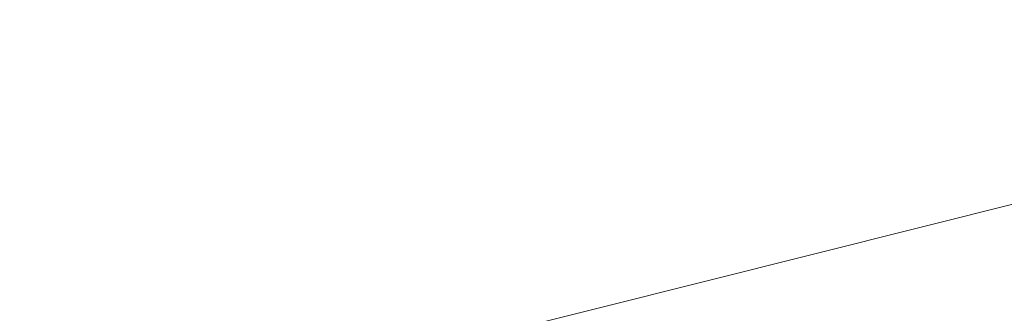
# Model space of a CAD drawing. Units: inches. Extents: x 2091 to 2899, y 967 to 2217.
# Tile 99 of 256: x 2251.243 to 2252.382, y 1100.071 to 1100.41. Entities that reach past the tile are written whole.
import ezdxf

# ---------------------------------------------------------------- set-up
doc = ezdxf.new("R2010")
doc.units = ezdxf.units.IN
doc.layers.add('A-ANNO-DIMS', color=2, linetype='Continuous', lineweight=18)
doc.layers.add('L-PLNT-TREE', color=94, linetype='Continuous', lineweight=13)
doc.layers.add('A-WALL-PATT', color=141, linetype='Continuous', lineweight=13, true_color=0xadddf7)
doc.styles.get("Standard").update_dxf_attribs({"font": 'arial.ttf'})
doc.dimstyles.new('ISO-25', dxfattribs={"dimtxt": 4, "dimasz": 4, "dimexe": 1.25, "dimexo": 0.625, "dimtad": 1, "dimdec": 0, "dimlunit": 3, "dimtxsty": 'Standard', "dimcen": 2.5, "dimadec": 0, "dimazin": 0, "dimtfac": 1, "dimtdec": 0, "dimtmove": 0, "dimatfit": 3, "dimfxl": 1, "dimarcsym": 0})

# ---------------------------------------------------------------- blocks, each defined once
blk = doc.blocks.new('*U29')
blk.add_line((-402.336, 12.192), (-451.104, 0))
blk = doc.blocks.new('*D71')
at = {"layer": 'A-ANNO-DIMS', "color": 0, "lineweight": -2, "transparency": 16777216}
for p, q in [((2212.1436, 1351.2941), (2212.1436, 969.4643)), ((2452.1436, 1351.2941), (2452.1436, 969.4643)), ((2216.1436, 970.7143), (2448.1436, 970.7143))]:
    blk.add_line(p, q, dxfattribs=at)
at = {"layer": 'A-ANNO-DIMS', "color": 0, "transparency": 16777216}
for points in [[(2216.1436, 971.381), (2216.1436, 970.0476), (2212.1436, 970.7143)], [(2448.1436, 971.381), (2448.1436, 970.0476), (2452.1436, 970.7143)]]:
    blk.add_solid(points, dxfattribs=at)
at = {"layer": 'Defpoints', "color": 0, "transparency": 16777216}
for p in [(2212.1436, 1351.9191), (2452.1436, 1351.9191), (2452.1436, 970.7143)]:
    blk.add_point(p, dxfattribs=at)
at = {"layer": 'A-ANNO-DIMS', "color": 0, "transparency": 16777216, "insert": (2332.1436, 973.3816), "char_height": 4, "attachment_point": 5}
blk.add_mtext('20\'-0"', dxfattribs=at)
blk = doc.blocks.new('*D75')
at = {"layer": 'A-ANNO-DIMS', "color": 0, "lineweight": -2, "transparency": 16777216}
for p, q in [((2212.1436, 1274.7941), (2212.1436, 969.4643)), ((2308.1436, 1274.7941), (2308.1436, 969.4643)), ((2216.1436, 970.7143), (2304.1436, 970.7143))]:
    blk.add_line(p, q, dxfattribs=at)
at = {"layer": 'A-ANNO-DIMS', "color": 0, "transparency": 16777216}
for points in [[(2216.1436, 971.381), (2216.1436, 970.0476), (2212.1436, 970.7143)], [(2304.1436, 971.381), (2304.1436, 970.0476), (2308.1436, 970.7143)]]:
    blk.add_solid(points, dxfattribs=at)
at = {"layer": 'Defpoints', "color": 0, "transparency": 16777216}
for p in [(2212.1436, 1275.4191), (2308.1436, 1275.4191), (2308.1436, 970.7143)]:
    blk.add_point(p, dxfattribs=at)
at = {"layer": 'A-ANNO-DIMS', "color": 0, "transparency": 16777216, "insert": (2260.1436, 973.3816), "char_height": 4, "attachment_point": 5}
blk.add_mtext('8\'-0"', dxfattribs=at)

msp = doc.modelspace()

# ---------------------------------------------------------------- hatches: boundary and pattern name
at = {"layer": 'A-WALL-PATT'}
h = msp.add_hatch(color=256, dxfattribs=at)
h.dxf.hatch_style = 1
h.paths.add_polyline_path([(2803.1436, 2050.9191), (2203.1436, 2050.9191), (2203.1436, 1090.9191), (2803.1436, 1090.9191)])
h.paths.add_polyline_path([(2635.7989, 1147.5405), (2674.5241, 1147.5405, 0.376086), (2678.5297, 1152.8802), (2678.5297, 1159.5565, 0.333335), (2674.5243, 1163.5618), (2674.5243, 1163.5619), (2674.5243, 1192.9344), (2635.806, 1192.9344), (2597.0876, 1192.9344), (2597.0876, 1163.5618, 0.333335), (2593.0823, 1159.5565), (2593.0823, 1152.8802, 0.376086), (2597.0879, 1147.5405)], flags=0)
h.paths.add_polyline_path([(2436.0104, 1278.2408, 0.000483), (2435.9526, 1278.215, -0.001328), (2435.9356, 1278.1117, -0.001711), (2436.1164, 1278.0408, 0.002185)], flags=0)
h.paths.add_polyline_path([(2794.1436, 1143.4191), (2794.1436, 1347.4191), (2543.3702, 1347.4191), (2543.3702, 1351.9191), (2794.1436, 1351.9191), (2794.1436, 1392.7136), (2793.9474, 1392.7136), (2793.9474, 1473.5369), (2794.1436, 1473.5369), (2794.1436, 1531.9191), (2650.1436, 1531.9191), (2650.1436, 1536.4191), (2794.1436, 1536.4191), (2794.1436, 1692.4191), (2609.3756, 1692.4191), (2609.3756, 1644.4191), (2604.8756, 1644.4191), (2604.8756, 1744.9191), (2609.3756, 1744.9191), (2609.3756, 1696.9191), (2794.1436, 1696.9191), (2794.1436, 1780.9191), (2609.6436, 1780.9191), (2493.8756, 1780.9191), (2493.8756, 1785.4191), (2609.6436, 1785.4191), (2794.1436, 1785.4191), (2794.1436, 1847.9388), (2793.9512, 1847.9388), (2793.9512, 1928.7622), (2794.1436, 1928.7622), (2794.1436, 1941.4191), (2614.1436, 1941.4191), (2614.1436, 1821.4191), (2609.6436, 1821.4191), (2609.6436, 1941.4191), (2392.1436, 1941.4191), (2392.1436, 1819.9191), (2387.6436, 1819.9191), (2387.6436, 1941.4191), (2212.1436, 1941.4191), (2212.1436, 1783.9191), (2392.1436, 1783.9191), (2392.1436, 1780.9191), (2212.1436, 1780.9191), (2212.1436, 1629.4191), (2387.6436, 1629.4191), (2387.6436, 1744.9191), (2392.1436, 1744.9191), (2392.1436, 1627.9191), (2317.1436, 1627.9191), (2317.1436, 1551.4191), (2317.1436, 1536.4191), (2459.3836, 1536.4191), (2459.3836, 1602.3965), (2463.8836, 1602.3965), (2463.8836, 1531.9191), (2456.6436, 1531.9191), (2456.6436, 1529.9191), (2452.1436, 1529.9191), (2452.1436, 1531.9191), (2312.6436, 1531.9191), (2312.6436, 1551.4191), (2306.1436, 1551.4191), (2306.1436, 1555.9191), (2308.1436, 1555.9191), (2308.1436, 1551.4191), (2312.6436, 1551.4191), (2312.6436, 1627.9191), (2212.1436, 1627.9191), (2212.1436, 1555.9191), (2270.1436, 1555.9191), (2270.1436, 1551.4191), (2212.1436, 1551.4191), (2212.1436, 1351.9191), (2272.1436, 1351.9191), (2272.1436, 1347.4191), (2212.1436, 1347.4191), (2212.1436, 1275.4191), (2308.1436, 1275.4191), (2308.1436, 1351.9191), (2452.1436, 1351.9191), (2452.1436, 1493.9191), (2456.6436, 1493.9191), (2456.6436, 1347.4191), (2312.6436, 1347.4191), (2312.6436, 1270.9191), (2212.1436, 1270.9191), (2212.1436, 1099.9191), (2281.2375, 1099.9191), (2282.871, 1110.9138), (2282.0083, 1116.9966), (2278.5577, 1121.4204), (2268.2056, 1128.0562), (2272.0876, 1128.0562), (2273.8129, 1131.927), (2279.4203, 1134.6919), (2285.0278, 1135.2449), (2287.6158, 1137.4568), (2288.0471, 1138.0098), (2289.3411, 1140.7747), (2291.0665, 1139.6687), (2292.3605, 1135.2449), (2295.3798, 1136.9038), (2296.2425, 1135.7979), (2297.1052, 1133.033), (2300.1246, 1138.0098), (2303.1439, 1138.0098), (2304.4379, 1135.7979), (2303.1439, 1133.586), (2306.5946, 1134.6919), (2307.8887, 1133.033), (2310.908, 1135.2449), (2313.9274, 1134.1389), (2315.6269, 1132.4271), (2308.32, 1117.5496), (2290.2038, 1109.8079), (2288.9098, 1103.1721), (2289.2723, 1099.9191), (2434.9182, 1099.9191), (2431.5932, 1124.7881), (2429.9302, 1169.5531), (2430.9272, 1240.5197), (2435.6589, 1238.1861), (2437.1352, 1196.5541), (2438.7982, 1143.9731), (2442.6782, 1111.9981), (2446.5582, 1099.9191), (2794.1436, 1099.9191), (2794.1436, 1138.9191), (2548.0324, 1138.9191), (2548.0324, 1143.4191), (2548.0324, 1148.8191), (2546.6685, 1148.0316), (2528.6857, 1179.1786, 0.256256), (2512.0324, 1148.8191), (2512.0324, 1143.4191), (2512.0324, 1138.9191), (2507.5324, 1138.9191), (2507.5324, 1143.4191), (2507.5324, 1148.8191, 0.256256), (2490.8792, 1179.1786), (2472.8964, 1148.0316), (2471.5324, 1148.8191), (2471.5324, 1143.4191), (2467.0324, 1143.4191), (2467.0324, 1269.9458, 0.039061), (2460.91, 1273.5801), (2467.0324, 1273.5801), (2467.0324, 1286.3254, 0.014511), (2465.2162, 1286.7619), (2467.0324, 1287.0526), (2467.0324, 1323.4191), (2471.5324, 1323.4191), (2471.5324, 1148.8191), (2489.5324, 1179.996), (2490.8964, 1179.2085), (2490.8792, 1179.1786, -0.256256), (2507.5324, 1148.8191), (2507.5324, 1143.4191), (2512.0324, 1143.4191), (2512.0324, 1148.8191, -0.256256), (2528.6857, 1179.1786), (2528.6685, 1179.2085), (2530.0324, 1179.996), (2548.0324, 1148.8191), (2548.0324, 1143.4191)], flags=16)
h.paths.add_polyline_path([(2607.7685, 1200.9451), (2607.7685, 1265.0306), (2597.0876, 1281.052), (2619.7846, 1281.052), (2627.7953, 1337.1269), (2635.7989, 1337.1269), (2643.8167, 1337.1269), (2651.8274, 1281.052), (2674.5243, 1281.052), (2663.8434, 1265.0306), (2663.8434, 1200.9451), (2635.806, 1200.9451)], flags=0)
edge = h.paths.add_edge_path(flags=0)
edge.add_ellipse((13303.8962, 1272.9987), major_axis=(-10595.313, 0), ratio=0.8423038701, start_angle=0.62823722, end_angle=0.6465541, ccw=False)
edge.add_ellipse((2711.7004, 1156.8527), major_axis=(2.2198, 0), ratio=0.842304, start_angle=111.5352, end_angle=180.6282, ccw=False)
edge.add_ellipse((13303.1563, 1272.9987), major_axis=(-10593.0263, 0), ratio=0.8423038695, start_angle=0.52827147, end_angle=0.6465541, ccw=False)
edge.add_line((2710.7646, 1175.3333), (2710.13, 1175.3333))
edge.add_ellipse((2710.13, 1176.5798), major_axis=(1.4798, 0), ratio=0.842304, start_angle=180, end_angle=270, ccw=False)
edge.add_line((2708.6501, 1176.5798), (2708.6501, 1200.7829))
edge.add_ellipse((2710.13, 1200.7829), major_axis=(1.4798, 0), ratio=0.842304, start_angle=90, end_angle=180, ccw=False)
edge.add_line((2710.13, 1202.0294), (2710.4651, 1202.0294))
edge.add_ellipse((13303.1563, 1272.9987), major_axis=(-10593.0263, 0), ratio=0.8423038695, start_angle=-0.09022909, end_angle=0.38386678, ccw=False)
edge.add_ellipse((2710.13, 1290.927), major_axis=(-1.4798, 0), ratio=0.842304, start_angle=0, end_angle=90, ccw=False)
edge.add_line((2708.6501, 1290.927), (2708.6501, 1315.1302))
edge.add_ellipse((2710.13, 1315.1302), major_axis=(-1.4798, 0), ratio=0.842304, start_angle=-90, end_angle=0, ccw=False)
edge.add_line((2710.13, 1316.3767), (2710.7063, 1316.3767))
edge.add_ellipse((3238.4017, 1296.2896), major_axis=(528.234, 0), ratio=0.84230387, start_angle=176.349572, end_angle=177.82005, ccw=False)
edge.add_ellipse((2775.063, 1071.4507), major_axis=(313.3078, 0), ratio=0.84230387, start_angle=102.125966, end_angle=103.780529, ccw=False)
edge.add_ellipse((2775.063, 1078.3057), major_axis=(-305.3029, 0), ratio=0.84230387, start_angle=-79.790461, end_angle=-77.555373, ccw=False)
edge.add_ellipse((2695.1418, 1541.9754), major_axis=(-250.9602, 0), ratio=0.84230387, start_angle=99.256566, end_angle=102.554933)
edge.add_line((2741.4103, 1334.2143), (2747.1325, 1337.3785))
edge.add_ellipse((2747.5386, 1336.8575), major_axis=(-0.7399, 0), ratio=0.842304, start_angle=270, end_angle=307.9331, ccw=False)
edge.add_ellipse((2747.5386, 1336.8575), major_axis=(-0.7399, 0), ratio=0.842304, start_angle=232.0669, end_angle=270, ccw=False)
edge.add_line((2747.9447, 1337.3785), (2753.6669, 1334.2143))
edge.add_ellipse((2799.9355, 1541.9754), major_axis=(250.9602, 0), ratio=0.84230387, start_angle=257.445067, end_angle=260.743434)
edge.add_ellipse((2720.0142, 1078.3057), major_axis=(305.3029, 0), ratio=0.84230387, start_angle=77.555373, end_angle=79.790461, ccw=False)
edge.add_ellipse((2720.0142, 1071.4507), major_axis=(-313.3078, 0), ratio=0.84230387, start_angle=256.219471, end_angle=257.874034, ccw=False)
edge.add_ellipse((2256.6755, 1296.2896), major_axis=(-528.234, 0), ratio=0.84230387, start_angle=182.17995, end_angle=183.650428, ccw=False)
edge.add_line((2784.3709, 1316.3767), (2784.9472, 1316.3767))
edge.add_ellipse((2784.9472, 1315.1302), major_axis=(1.4798, 0), ratio=0.842304, start_angle=0, end_angle=90, ccw=False)
edge.add_line((2786.4271, 1315.1302), (2786.4271, 1290.927))
edge.add_ellipse((2784.9472, 1290.927), major_axis=(1.4798, 0), ratio=0.842304, start_angle=270, end_angle=360, ccw=False)
edge.add_ellipse((-7808.0791, 1272.9987), major_axis=(10593.0263, 0), ratio=0.8423038695, start_angle=-0.38386678, end_angle=0.09022909, ccw=False)
edge.add_line((2784.6122, 1202.0294), (2784.9472, 1202.0294))
edge.add_ellipse((2784.9472, 1200.7829), major_axis=(1.4798, 0), ratio=0.842304, start_angle=0, end_angle=90, ccw=False)
edge.add_line((2786.4271, 1200.7829), (2786.4271, 1176.5798))
edge.add_ellipse((2784.9472, 1176.5798), major_axis=(-1.4798, 0), ratio=0.842304, start_angle=90, end_angle=180, ccw=False)
edge.add_line((2784.9472, 1175.3333), (2784.3126, 1175.3333))
edge.add_ellipse((-7808.0791, 1272.9987), major_axis=(10593.0263, 0), ratio=0.8423038695, start_angle=-0.6186432, end_angle=-0.52827147, ccw=False)
edge.add_ellipse((2783.3768, 1156.8527), major_axis=(-2.2198, 0), ratio=0.842304, start_angle=179.3718, end_angle=248.4648, ccw=False)
edge.add_ellipse((-7808.819, 1272.9987), major_axis=(-10595.313, 0), ratio=0.8423038658, start_angle=179.35344592, end_angle=179.3717628, ccw=False)
edge.add_ellipse((2780.2973, 1153.5008), major_axis=(-5.2464, 0), ratio=0.842304, start_angle=90, end_angle=179.3534, ccw=False)
edge.add_line((2780.2973, 1149.0817), (2714.7799, 1149.0817))
edge.add_ellipse((2714.7799, 1153.5008), major_axis=(5.2464, 0), ratio=0.842304, start_angle=180.6466, end_angle=270, ccw=False)
edge = h.paths.add_edge_path(flags=0)
edge.add_line((2718.1874, 1151.0078), (2718.1874, 1170.4724))
edge.add_ellipse((2721.1471, 1170.4724), major_axis=(-2.9597, 0), ratio=0.842304, start_angle=-90, end_angle=0, ccw=False)
edge.add_line((2721.1471, 1172.9653), (2773.9302, 1172.9653))
edge.add_ellipse((2773.9302, 1170.4724), major_axis=(-2.9597, 0), ratio=0.842304, start_angle=180, end_angle=270, ccw=False)
edge.add_line((2776.8899, 1170.4724), (2776.8899, 1151.0078))
edge.add_line((2776.8899, 1151.0078), (2718.1874, 1151.0078))
edge = h.paths.add_edge_path(flags=0)
edge.add_line((2718.1874, 1180.2342), (2718.1874, 1199.0578))
edge.add_ellipse((2747.5386, 1320.3986), major_axis=(147.0179, 0), ratio=0.84230387, start_angle=256.401865, end_angle=283.598135)
edge.add_line((2776.8899, 1199.0578), (2776.8899, 1180.2342))
edge.add_ellipse((2747.5386, 1301.575), major_axis=(147.0179, 0), ratio=0.84230387, start_angle=256.401865, end_angle=283.598135, ccw=False)
edge = h.paths.add_edge_path(flags=0)
edge.add_ellipse((13303.1563, 1272.9987), major_axis=(-10591.5465, 0), ratio=0.8423038696, start_angle=0.05559431, end_angle=0.37776419, ccw=False)
edge.add_line((2711.6169, 1262.7217), (2715.6674, 1249.4954))
edge.add_ellipse((6413.892, 1241.6919), major_axis=(-3698.2362, 0), ratio=0.84230387, start_angle=-0.1208974, end_angle=0.3640763)
edge.add_line((2715.761, 1218.1925), (2711.9343, 1203.1674))
edge = h.paths.add_edge_path(flags=0)
edge.add_line((2718.1874, 1251.0746), (2716.0025, 1267.4504))
edge.add_ellipse((2742.1512, 1202.1895), major_axis=(81.7726, 0), ratio=0.8423039, start_angle=94.277421, end_angle=111.834954, ccw=False)
edge.add_line((2737.0097, 1270.9306), (2758.0675, 1270.9306))
edge.add_ellipse((2752.9261, 1202.1895), major_axis=(81.7726, 0), ratio=0.8423039, start_angle=68.165046, end_angle=85.722579, ccw=False)
edge.add_line((2779.0747, 1267.4504), (2776.8899, 1251.0746))
edge.add_ellipse((2750.3381, 1187.8854), major_axis=(79.5797, 0), ratio=0.8423039, start_angle=67.208085, end_angle=85.12993)
edge.add_line((2756.0347, 1254.7437), (2739.0426, 1254.7437))
edge.add_ellipse((2744.7392, 1187.8854), major_axis=(79.5797, 0), ratio=0.8423039, start_angle=94.87007, end_angle=112.791915)
edge = h.paths.add_edge_path(flags=0)
edge.add_line((2783.1429, 1203.1674), (2779.3162, 1218.1925))
edge.add_ellipse((-918.8147, 1241.6919), major_axis=(3698.2362, 0), ratio=0.84230387, start_angle=-0.3640763, end_angle=0.1208974)
edge.add_line((2779.4098, 1249.4954), (2783.4604, 1262.7217))
edge.add_ellipse((-7808.0791, 1272.9987), major_axis=(-10591.5465, 0), ratio=0.8423038695, start_angle=179.62223581, end_angle=179.94440569, ccw=False)
edge = h.paths.add_edge_path(flags=0)
edge.add_ellipse((2734.2009, 1286.6904), major_axis=(-0.3566, 6.3401), ratio=0.603834, start_angle=89.00201, end_angle=253.65741, ccw=False)
edge.add_line((2730.369, 1286.5418), (2730.369, 1301.352))
edge.add_line((2730.369, 1301.352), (2735.9133, 1305.2148))
edge.add_ellipse((2736.3849, 1304.7346), major_axis=(0.7399, 0), ratio=0.842304, start_angle=90, end_angle=134.4802, ccw=False)
edge.add_line((2736.3849, 1305.3578), (2738.0328, 1305.3578))
edge.add_line((2738.0328, 1305.3578), (2738.0328, 1307.7079))
edge.add_ellipse((2794.2016, 1307.7079), major_axis=(56.1689, 0), ratio=0.8423039, start_angle=150.56143, end_angle=180, ccw=False)
edge.add_ellipse((2700.8756, 1307.7079), major_axis=(-56.1689, 0), ratio=0.8423039, start_angle=180, end_angle=209.43857, ccw=False)
edge.add_line((2757.0444, 1307.7079), (2757.0444, 1305.3578))
edge.add_line((2757.0444, 1305.3578), (2758.6923, 1305.3578))
edge.add_ellipse((2758.6923, 1304.7346), major_axis=(-0.7399, 0), ratio=0.842304, start_angle=225.5198, end_angle=270, ccw=False)
edge.add_line((2759.1639, 1305.2148), (2764.7082, 1301.352))
edge.add_line((2764.7082, 1301.352), (2764.7082, 1286.5418))
edge.add_ellipse((2760.8763, 1286.6904), major_axis=(0.3566, 6.3401), ratio=0.603834, start_angle=106.34259, end_angle=270.99799, ccw=False)
edge.add_line((2757.0444, 1285.7971), (2757.0444, 1307.7079))
edge.add_ellipse((2700.8756, 1307.7079), major_axis=(-56.1689, 0), ratio=0.8423039, start_angle=180, end_angle=209.43857)
edge.add_ellipse((2794.2016, 1307.7079), major_axis=(56.1689, 0), ratio=0.8423039, start_angle=150.56143, end_angle=180)
edge.add_line((2738.0328, 1307.7079), (2738.0328, 1285.7971))
h.paths.add_polyline_path([(2417.8123, 1104.4497), (2413.4923, 1102.5297), (2410.6123, 1103.9697), (2409.1723, 1106.3697), (2407.2523, 1107.3297), (2406.2923, 1109.7297), (2405.3323, 1114.0497), (2405.3323, 1117.8897), (2406.2923, 1120.1297), (2407.2523, 1119.8097), (2408.8483, 1118.3277), (2410.1739, 1119.4242), (2410.2113, 1120.4057), (2411.0407, 1121.4191), (2410.6993, 1119.8587), (2410.1739, 1119.4242), (2410.0885, 1117.1761), (2411.1328, 1116.2063), (2413.9723, 1119.3297), (2416.8523, 1120.7697), (2416.8697, 1120.7988), (2417.0351, 1119.4051), (2417.8962, 1118.1434), (2418.2923, 1118.3697), (2419.5444, 1120.0393), (2419.3609, 1118.3875), (2419.0321, 1119.3562), (2418.3989, 1118.5119), (2419.2523, 1114.5297), (2418.7941, 1107.1988)], flags=0)
h.paths.add_polyline_path([(2508.8702, 1347.4191), (2508.3702, 1347.4191), (2508.3702, 1351.9191), (2508.8702, 1351.9191)], flags=0)
h.paths.add_polyline_path([(2473.3702, 1347.4191), (2472.3702, 1347.4191), (2467.8702, 1347.4191), (2467.8702, 1455.4191), (2472.3702, 1455.4191), (2472.3702, 1352.4191), (2473.3702, 1352.4191)], flags=0)
h.paths.add_polyline_path([(2352.1062, 1217.4462), (2349.2262, 1218.8862), (2347.7862, 1221.2862), (2345.8662, 1222.2462), (2344.9062, 1224.6462), (2343.9462, 1228.9662), (2343.9462, 1232.8062), (2344.9062, 1235.0462), (2345.8662, 1234.7262), (2347.4623, 1233.2442), (2348.7879, 1234.3407), (2348.8252, 1235.3222), (2349.6547, 1236.3355), (2349.3132, 1234.7752), (2348.7879, 1234.3407), (2348.7024, 1232.0926), (2349.7468, 1231.1228), (2352.5862, 1234.2462), (2355.4662, 1235.6862), (2355.4837, 1235.7153), (2355.649, 1234.3216), (2356.5102, 1233.0599), (2356.9062, 1233.2862), (2358.1584, 1234.9558), (2357.9749, 1233.304), (2357.6461, 1234.2726), (2357.0129, 1233.4284), (2357.8662, 1229.4462), (2357.4081, 1222.1153), (2356.4262, 1219.3662)], flags=0)
h.paths.add_polyline_path([(2348.2968, 1112.2244), (2347.0138, 1112.3104), (2345.5298, 1114.1274), (2345.7318, 1115.8584), (2346.8118, 1116.9824), (2346.8118, 1114.6464), (2345.8668, 1114.2144), (2346.8798, 1114.3004)], flags=0)
h.paths.add_polyline_path([(2347.0138, 1110.9264), (2346.2718, 1110.4934), (2346.6098, 1111.1864)], flags=0)
h.paths.add_polyline_path([(2345.8668, 1118.1944), (2345.5298, 1117.3294), (2343.7078, 1118.0214), (2344.3828, 1118.6264)], flags=0)
h.paths.add_polyline_path([(2346.6768, 1109.2824), (2346.0698, 1108.0714), (2345.8668, 1110.0614)], flags=0)
h.paths.add_polyline_path([(2345.0568, 1119.7514), (2343.6398, 1119.7514), (2343.9778, 1121.1354)], flags=0)
h.paths.add_polyline_path([(2345.2598, 1116.5504), (2345.1248, 1115.8584), (2344.9218, 1115.6854), (2344.7198, 1116.3774)], flags=0)
h.paths.add_polyline_path([(2345.6648, 1112.3104), (2345.4618, 1111.5324), (2344.0448, 1111.9644), (2344.6518, 1112.5704)], flags=0)
h.paths.add_polyline_path([(2345.1918, 1113.3494), (2344.4498, 1113.8684), (2344.7198, 1114.3874)], flags=0)
h.paths.add_polyline_path([(2344.6518, 1116.8094), (2344.1798, 1115.6854), (2344.6518, 1115.3394), (2343.9098, 1114.9064), (2343.0328, 1115.9444), (2343.6398, 1116.4634)], flags=0)
h.paths.add_polyline_path([(2345.8668, 1106.6864), (2344.9898, 1105.5624), (2344.5168, 1106.6004)], flags=0)
h.paths.add_polyline_path([(2344.8548, 1110.0614), (2344.5168, 1109.2824), (2344.1128, 1109.7154)], flags=0)
h.paths.add_polyline_path([(2344.0448, 1113.5224), (2343.4378, 1113.0894), (2342.7628, 1113.9544)], flags=0)
h.paths.add_polyline_path([(2344.3148, 1111.0124), (2342.9648, 1110.3204), (2342.9648, 1111.0994)], flags=0)
h.paths.add_polyline_path([(2345.1248, 1104.6974), (2344.5848, 1103.7454), (2344.4498, 1104.2644)], flags=0)
h.paths.add_polyline_path([(2342.8298, 1121.2224), (2341.7498, 1120.5304), (2340.5358, 1121.0494), (2340.1308, 1121.8284), (2340.6708, 1122.9524), (2341.1428, 1121.8284), (2341.6148, 1122.0014)], flags=0)
h.paths.add_polyline_path([(2342.9648, 1119.7514), (2343.0328, 1118.4534), (2342.0878, 1118.0214), (2342.0198, 1119.4914)], flags=0)
h.paths.add_polyline_path([(2342.6948, 1116.8964), (2341.9528, 1116.6364), (2342.0198, 1117.3294)], flags=0)
h.paths.add_polyline_path([(2343.0328, 1112.2244), (2342.0198, 1111.7914), (2341.5478, 1112.2244), (2342.3578, 1113.3494)], flags=0)
h.paths.add_polyline_path([(2343.7748, 1104.4374), (2342.6278, 1102.8804), (2342.6948, 1104.6104), (2343.4378, 1105.1294)], flags=0)
h.paths.add_polyline_path([(2342.0198, 1115.0794), (2340.8058, 1115.5124), (2340.9408, 1116.3774)], flags=0)
h.paths.add_polyline_path([(2341.4808, 1120.0974), (2341.4808, 1119.4054), (2341.0758, 1119.5784), (2341.1428, 1120.0974)], flags=0)
h.paths.add_polyline_path([(2341.8178, 1114.4734), (2340.9408, 1113.0894), (2340.8058, 1114.5604)], flags=0)
h.paths.add_polyline_path([(2341.1428, 1118.5404), (2340.9408, 1116.9824), (2339.0508, 1117.6754), (2339.0508, 1118.6264)], flags=0)
h.paths.add_polyline_path([(2342.6948, 1101.6684), (2341.9528, 1101.8414), (2342.5598, 1102.3614)], flags=0)
h.paths.add_polyline_path([(2340.3328, 1119.6654), (2338.4438, 1119.5784), (2337.9038, 1120.3574), (2339.6578, 1120.6164)], flags=0)
h.paths.add_polyline_path([(2340.3328, 1115.3394), (2340.0628, 1113.6954), (2339.3878, 1115.3394)], flags=0)
h.paths.add_polyline_path([(2341.8178, 1103.8314), (2341.5478, 1102.8804), (2341.1428, 1103.6584)], flags=0)
h.paths.add_polyline_path([(2339.0508, 1122.8664), (2337.2958, 1121.8284), (2337.0938, 1123.1254), (2337.7688, 1123.8184)], flags=0)
h.paths.add_polyline_path([(2339.1178, 1121.7414), (2338.8478, 1121.2224), (2338.1738, 1121.0494), (2338.3758, 1121.5684)], flags=0)
h.paths.add_polyline_path([(2339.1858, 1119.3194), (2338.6458, 1118.7134), (2338.2408, 1118.1074), (2338.2408, 1118.8864)], flags=0)
h.paths.add_polyline_path([(2341.1428, 1101.9284), (2340.6028, 1101.2364), (2340.0628, 1101.8414), (2340.6028, 1102.3614)], flags=0)
h.paths.add_polyline_path([(2337.6338, 1117.7614), (2336.6208, 1118.2804), (2337.2958, 1118.9724)], flags=0)
h.paths.add_polyline_path([(2336.8238, 1119.5784), (2334.7988, 1118.9724), (2335.2038, 1120.3574), (2336.5538, 1120.8764)], flags=0)
h.paths.add_polyline_path([(2339.1178, 1100.4574), (2337.3638, 1100.5434), (2336.7558, 1101.2364)], flags=0)
h.paths.add_polyline_path([(2336.3508, 1122.4334), (2336.0138, 1121.9144), (2334.9338, 1122.4334), (2334.5288, 1123.4714), (2335.7438, 1122.7794)], flags=0)
h.paths.add_polyline_path([(2334.7318, 1120.8764), (2334.2588, 1120.3574), (2334.0568, 1120.7894), (2334.5968, 1121.3084)], flags=0)
h.paths.add_polyline_path([(2334.4618, 1122.1744), (2332.5718, 1121.3084), (2331.3568, 1122.1744), (2332.0998, 1122.8664)], flags=0)
h.paths.add_polyline_path([(2334.2588, 1118.5404), (2333.3818, 1118.4534), (2333.6518, 1119.3194)], flags=0)
h.paths.add_polyline_path([(2335.5418, 1102.2744), (2334.1918, 1102.6204), (2335.2718, 1103.3124)], flags=0)
h.paths.add_polyline_path([(2332.7068, 1119.6654), (2331.6948, 1120.4434), (2332.5048, 1120.7894)], flags=0)
h.paths.add_polyline_path([(2334.7318, 1101.1494), (2333.5168, 1101.5824), (2333.9888, 1101.7554)], flags=0)
h.paths.add_polyline_path([(2332.6398, 1116.6364), (2331.0868, 1116.2904), (2331.9648, 1118.1944)], flags=0)
h.paths.add_polyline_path([(2330.7498, 1121.5684), (2330.2768, 1120.2704), (2328.5228, 1119.3194), (2328.9948, 1121.0494)], flags=0)
h.paths.add_polyline_path([(2330.7498, 1118.6264), (2330.0078, 1117.5024), (2329.8728, 1118.0214)], flags=0)
h.paths.add_polyline_path([(2332.0998, 1102.3614), (2330.5468, 1102.0144), (2331.6948, 1102.9664)], flags=0)
h.paths.add_polyline_path([(2329.5348, 1113.6084), (2329.0628, 1112.3104), (2328.5898, 1113.3494)], flags=0)
h.paths.add_polyline_path([(2328.3878, 1117.8484), (2327.5098, 1116.5504), (2327.1728, 1117.7614)], flags=0)
h.paths.add_polyline_path([(2329.7378, 1106.5134), (2329.5348, 1105.3024), (2328.2528, 1106.0814)], flags=0)
h.paths.add_polyline_path([(2328.6578, 1114.3874), (2328.0498, 1114.1274), (2328.3198, 1114.9064)], flags=0)
h.paths.add_polyline_path([(2328.3198, 1112.2244), (2327.1058, 1112.1374), (2326.7008, 1112.6564)], flags=0)
h.paths.add_polyline_path([(2326.9028, 1115.2524), (2326.7008, 1114.1274), (2325.2158, 1113.6084), (2326.0928, 1115.3394)], flags=0)
h.paths.add_polyline_path([(2326.6328, 1108.3304), (2326.0928, 1107.3794), (2325.8908, 1108.5034), (2326.4978, 1109.1094)], flags=0)
h.paths.add_polyline_path([(2615.1436, 1531.9191), (2609.6436, 1531.9191), (2609.6436, 1620.4191), (2614.1436, 1620.4191), (2614.1436, 1536.4191), (2615.1436, 1536.4191)], flags=0)
h.paths.add_polyline_path([(2545.1436, 1563.4191), (2464.1436, 1563.4191), (2464.1436, 1632.4191), (2509.1436, 1632.4191), (2509.1436, 1627.9191), (2509.1436, 1603.9191), (2468.6436, 1603.9191), (2468.6436, 1567.9191), (2540.6436, 1567.9191), (2540.6436, 1591.9191), (2545.1436, 1591.9191)], flags=0)
h.paths.add_polyline_path([(2388.969, 1549.9857), (2357.4342, 1549.9857), (2357.4342, 1623.3608), (2399.3628, 1623.3608), (2435.6895, 1623.3608), (2435.5925, 1602.5593), (2435.5925, 1602.3965), (2388.969, 1602.3965)], flags=0)
h.paths.add_polyline_path([(2388.8806, 1555.8092), (2374.9044, 1555.8092), (2374.9044, 1600.5716), (2374.9044, 1615.4576), (2406.3509, 1615.4576), (2406.3509, 1618.9394), (2412.1743, 1615.4576), (2406.3509, 1611.9759), (2406.3509, 1615.4576), (2388.8806, 1615.4576)], flags=0)
h.paths.add_polyline_path([(2568.8756, 1644.4191), (2453.3756, 1644.4191), (2453.3756, 1785.4191), (2457.8756, 1785.4191), (2457.8756, 1648.9191), (2568.8756, 1648.9191)], flags=0)
h.paths.add_polyline_path([(2212.1436, 1945.9191), (2212.1436, 2041.9191), (2794.1436, 2041.9191), (2794.1436, 1945.9191)], flags=16)
h.paths.add_polyline_path([(2271.0827, 1964.3172), (2776.853, 1964.3172), (2776.853, 2037.1696), (2271.0827, 2037.1696)], flags=8)
h.paths.add_polyline_path([(2380.6493, 1536.8241), (2461.0408, 1536.8241), (2461.0408, 1554.6526), (2380.6493, 1554.6526)], flags=8)
h.paths.add_polyline_path([(2240.7557, 1609.7255), (2309.1858, 1609.7255), (2309.1858, 1617.6982), (2240.7557, 1617.6982)], flags=8)
h.paths.add_polyline_path([(2212.6773, 1313.5041), (2282.5915, 1313.5041), (2282.5915, 1322.7452), (2212.6773, 1322.7452)], flags=8)
h.paths.add_polyline_path([(2457.112, 1114.7786), (2558.4816, 1114.7786), (2558.4816, 1142.2197), (2457.112, 1142.2197)], flags=8)
h.paths.add_polyline_path([(2473.4423, 1273.0101), (2604.6412, 1273.0101), (2604.6412, 1318.3469), (2473.4423, 1318.3469)], flags=8)
h.paths.add_polyline_path([(2638.8763, 1626.9774), (2684.2504, 1627.9767), (2684.0385, 1637.5975), (2638.6644, 1636.5982)], flags=8)
h.paths.add_polyline_path([(2537.5906, 1453.7934), (2628.3895, 1453.7934), (2628.3895, 1475.3448), (2537.5906, 1475.3448)], flags=8)
h.paths.add_polyline_path([(2504.1376, 1714.6324), (2554.6472, 1714.6324), (2554.6472, 1730.2377), (2504.1376, 1730.2377)], flags=8)
h.paths.add_polyline_path([(2487.5012, 1575.6519), (2535.0971, 1575.6519), (2535.0971, 1598.3776), (2487.5012, 1598.3776)], flags=8)
h.paths.add_polyline_path([(2709.0994, 1735.7103), (2740.0166, 1735.7103), (2740.0166, 1749.9376), (2709.0994, 1749.9376)], flags=8)
h.paths.add_polyline_path([(2442.4384, 1792.1717), (2564.7288, 1792.1717), (2564.7288, 1842.0002), (2442.4384, 1842.0002)], flags=8)
h.paths.add_polyline_path([(2655.8158, 1809.6441), (2789.5201, 1806.6938), (2790.085, 1832.2916), (2656.3806, 1835.2419)], flags=8)
h.paths.add_polyline_path([(2234.8427, 1797.7201), (2368.5929, 1794.7689), (2369.1607, 1820.5041), (2235.4106, 1823.4554)], flags=8)
h.paths.add_polyline_path([(2245.1385, 1644.0063), (2398.4277, 1640.6239), (2398.9948, 1666.3248), (2245.7056, 1669.7073)], flags=8)
h.paths.add_polyline_path([(2306.1428, 1431.1685), (2413.7683, 1428.7937), (2414.3331, 1454.3915), (2306.7077, 1456.7664)], flags=8)
h.paths.add_polyline_path([(2306.8346, 1458.2331), (2393.3805, 1456.3234), (2393.9328, 1481.3544), (2307.3869, 1483.2641)], flags=8)

# ---------------------------------------------------------------- block references
at = {"layer": 'L-PLNT-TREE', "xscale": 0.0393700787401575, "yscale": 0.0393700787401575, "zscale": 0.0393700787401575}
msp.add_blockref('*U29', (2269.041, 1099.9191), dxfattribs=at)

# ---------------------------------------------------------------- dimensions: what is measured, and where the dimension line sits
at = {"layer": 'A-ANNO-DIMS'}
for base, p1, p2, picture, middle in [((2452.1436, 970.7143), (2212.1436, 1351.9191), (2452.1436, 1351.9191), '*D71', (2332.1436, 973.3816)), ((2308.1436, 970.7143), (2212.1436, 1275.4191), (2308.1436, 1275.4191), '*D75', (2260.1436, 973.3816))]:
    dim = msp.add_linear_dim(base=base, p1=p1, p2=p2, dimstyle='ISO-25', override={"dimdec": 1, "dimlfac": 1, "dimrnd": 0, "dimzin": 1, "dimdsep": 46, "dimlunit": 4, "dimfrac": 2}, dxfattribs=at)
    dim.commit()
    dim.dimension.update_dxf_attribs({"geometry": picture, "text_midpoint": middle})

doc.saveas('drawing.dxf')
